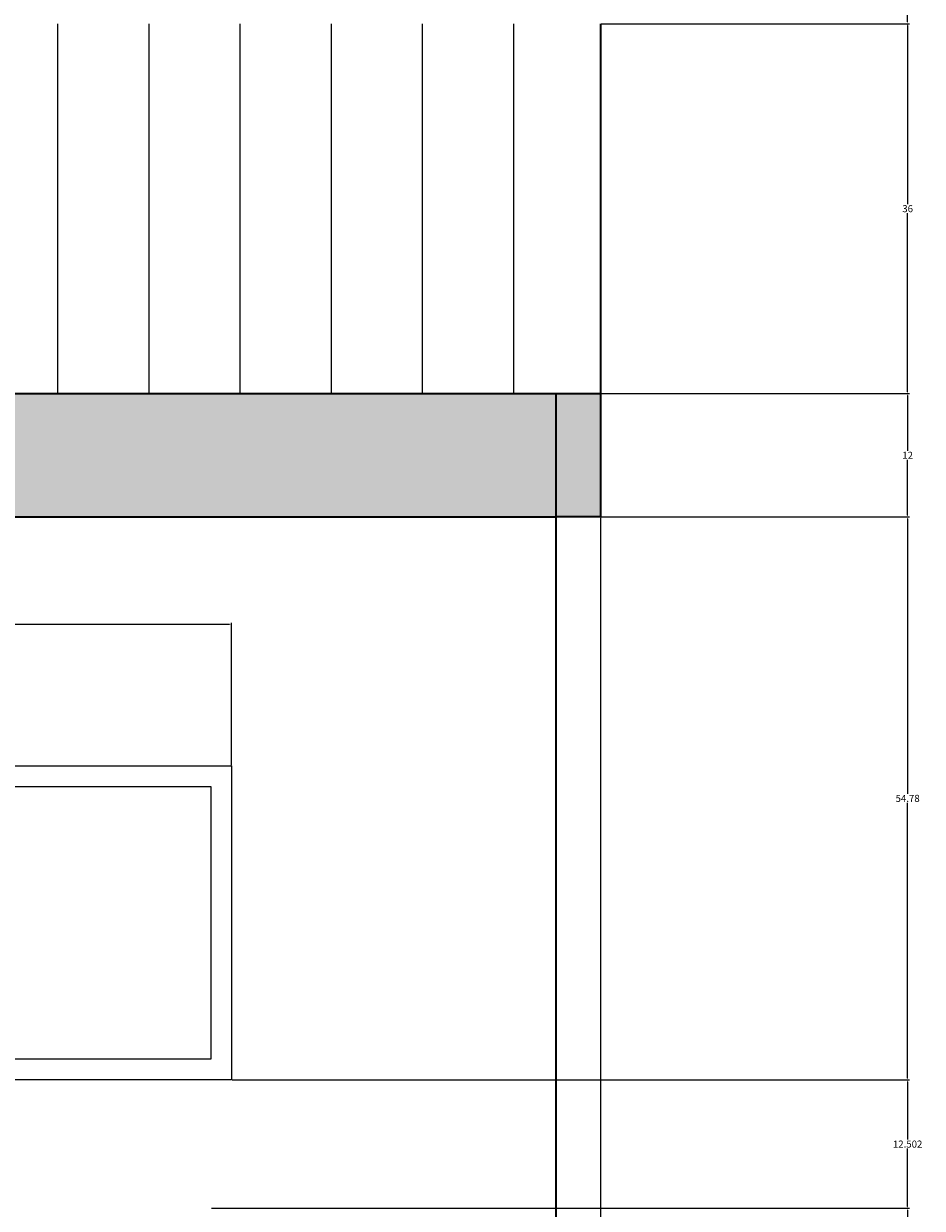
# Model space of a CAD drawing. Units: inches. Extents: x -145 to 510, y 5 to 386.
# Tile 24 of 25: x 423 to 510, y 157 to 272. Entities that reach past the tile are written whole.
import ezdxf

# ---------------------------------------------------------------- set-up
doc = ezdxf.new("R2010")
doc.units = ezdxf.units.IN
doc.header["$MEASUREMENT"] = 0
for name, color, linetype, lineweight in [('A-ANNO-DIMS', 2, 'Continuous', 18), ('A-ELEV', 7, 'Continuous', 35), ('A-ELEV-PATT', 8, 'Continuous', 13), ('A-GLAZ', 4, 'Continuous', 25)]:
    doc.layers.add(name, color=color, linetype=linetype, lineweight=lineweight)
doc.styles.get("Standard").update_dxf_attribs({"font": 'arial.ttf'})
doc.dimstyles.get("Standard").update_dxf_attribs({"dimtxt": 0.6875, "dimasz": 0.18, "dimexe": 0.18, "dimexo": 0.0625, "dimgap": 0.09, "dimtad": 0, "dimtih": 1, "dimtoh": 1, "dimdec": 4, "dimzin": 0, "dimdsep": 46, "dimlunit": 4, "dimtxsty": 'Standard', "dimcen": 0.09, "dimadec": 0, "dimazin": 0, "dimtfac": 1, "dimtdec": 4, "dimtofl": 0, "dimtmove": 0, "dimatfit": 3, "dimfxl": 1, "dimtolj": 1, "dimtzin": 0, "dimarcsym": 0})

# ---------------------------------------------------------------- blocks, each defined once
blk = doc.blocks.new('WIN-2200')
for points in [[(0, 30.55), (91.67, 30.55), (91.67, 0), (0, 0)], [(2, 28.55), (89.67, 28.55), (89.67, 2), (2, 2)]]:
    blk.add_lwpolyline(points, close=True)
blk = doc.blocks.new('*D5')
at = {"layer": 'A-ANNO-DIMS', "color": 0, "lineweight": -2, "transparency": 16777216}
for p, q in [((351.23, 199.73), (351.23, 213.6)), ((351.41, 213.42), (392.2, 213.42)), ((442.72, 213.42), (401.94, 213.42)), ((442.9, 199.73), (442.9, 213.6))]:
    blk.add_line(p, q, dxfattribs=at)
at = {"layer": 'A-ANNO-DIMS', "color": 0, "transparency": 16777216}
for points in [[(351.41, 213.45), (351.41, 213.39), (351.23, 213.42)], [(442.72, 213.45), (442.72, 213.39), (442.9, 213.42)]]:
    blk.add_solid(points, dxfattribs=at)
at = {"layer": 'Defpoints', "color": 0, "transparency": 16777216}
for p in [(442.9, 213.42), (351.23, 199.67), (442.9, 199.67)]:
    blk.add_point(p, dxfattribs=at)
at = {"layer": 'A-ANNO-DIMS', "color": 0, "transparency": 16777216, "insert": (397.07, 213.42), "char_height": 0.6875, "attachment_point": 5}
blk.add_mtext('\\A1;WINDOW W1 92 TYP.', dxfattribs=at)
blk = doc.blocks.new('*D19')
at = {"layer": 'A-ANNO-DIMS', "color": 0, "lineweight": -2, "transparency": 16777216}
for p, q in [((478.76, 355.89), (-144.05, 355.89)), ((-143.87, 355.71), (-143.87, 218.33)), ((-143.87, 80.07), (-143.87, 217.45)), ((-114.04, 79.89), (-144.05, 79.89))]:
    blk.add_line(p, q, dxfattribs=at)
at = {"layer": 'A-ANNO-DIMS', "color": 0, "transparency": 16777216}
for points in [[(-143.9, 355.71), (-143.84, 355.71), (-143.87, 355.89)], [(-143.9, 80.07), (-143.84, 80.07), (-143.87, 79.89)]]:
    blk.add_solid(points, dxfattribs=at)
at = {"layer": 'Defpoints', "color": 0, "transparency": 16777216}
for p in [(-143.87, 355.89), (478.83, 355.89), (-113.97, 79.89)]:
    blk.add_point(p, dxfattribs=at)
at = {"layer": 'A-ANNO-DIMS', "color": 0, "transparency": 16777216, "insert": (-143.87, 217.89), "char_height": 0.688, "attachment_point": 5}
blk.add_mtext('\\A1;276', dxfattribs=at)
blk = doc.blocks.new('*D32')
at = {"layer": 'A-ANNO-DIMS', "color": 0, "lineweight": -2, "transparency": 16777216}
for p, q in [((440.96, 156.61), (508.91, 156.61)), ((508.73, 156.43), (508.73, 136.37)), ((508.73, 115.44), (508.73, 135.49)), ((440.96, 115.26), (508.91, 115.26))]:
    blk.add_line(p, q, dxfattribs=at)
at = {"layer": 'A-ANNO-DIMS', "color": 0, "transparency": 16777216}
for points in [[(508.7, 156.43), (508.76, 156.43), (508.73, 156.61)], [(508.7, 115.44), (508.76, 115.44), (508.73, 115.26)]]:
    blk.add_solid(points, dxfattribs=at)
at = {"layer": 'Defpoints', "color": 0, "transparency": 16777216}
for p in [(440.9, 156.61), (508.73, 156.61), (440.9, 115.26)]:
    blk.add_point(p, dxfattribs=at)
at = {"layer": 'A-ANNO-DIMS', "color": 0, "transparency": 16777216, "insert": (508.73, 135.93), "char_height": 0.688, "attachment_point": 5}
blk.add_mtext('\\A1;41.35', dxfattribs=at)
blk = doc.blocks.new('*D33')
at = {"layer": 'A-ANNO-DIMS', "color": 0, "lineweight": -2, "transparency": 16777216}
for p, q in [((442.96, 169.11), (508.91, 169.11)), ((508.73, 168.93), (508.73, 163.3)), ((508.73, 156.79), (508.73, 162.42)), ((440.96, 156.61), (508.91, 156.61))]:
    blk.add_line(p, q, dxfattribs=at)
at = {"layer": 'A-ANNO-DIMS', "color": 0, "transparency": 16777216}
for points in [[(508.7, 168.93), (508.76, 168.93), (508.73, 169.11)], [(508.7, 156.79), (508.76, 156.79), (508.73, 156.61)]]:
    blk.add_solid(points, dxfattribs=at)
at = {"layer": 'Defpoints', "color": 0, "transparency": 16777216}
for p in [(442.9, 169.11), (508.73, 169.11), (440.9, 156.61)]:
    blk.add_point(p, dxfattribs=at)
at = {"layer": 'A-ANNO-DIMS', "color": 0, "transparency": 16777216, "insert": (508.73, 162.86), "char_height": 0.688, "attachment_point": 5}
blk.add_mtext('\\A1;12.502', dxfattribs=at)
blk = doc.blocks.new('*D34')
at = {"layer": 'A-ANNO-DIMS', "color": 0, "lineweight": -2, "transparency": 16777216}
for p, q in [((478.89, 223.89), (508.91, 223.89)), ((508.73, 223.71), (508.73, 196.94)), ((508.73, 169.29), (508.73, 196.06)), ((442.96, 169.11), (508.91, 169.11))]:
    blk.add_line(p, q, dxfattribs=at)
at = {"layer": 'A-ANNO-DIMS', "color": 0, "transparency": 16777216}
for points in [[(508.7, 223.71), (508.76, 223.71), (508.73, 223.89)], [(508.7, 169.29), (508.76, 169.29), (508.73, 169.11)]]:
    blk.add_solid(points, dxfattribs=at)
at = {"layer": 'Defpoints', "color": 0, "transparency": 16777216}
for p in [(478.83, 223.89), (508.73, 223.89), (442.9, 169.11)]:
    blk.add_point(p, dxfattribs=at)
at = {"layer": 'A-ANNO-DIMS', "color": 0, "transparency": 16777216, "insert": (508.73, 196.5), "char_height": 0.688, "attachment_point": 5}
blk.add_mtext('\\A1;54.78', dxfattribs=at)
blk = doc.blocks.new('*D35')
at = {"layer": 'A-ANNO-DIMS', "color": 0, "lineweight": -2, "transparency": 16777216}
for p, q in [((478.89, 235.89), (508.91, 235.89)), ((508.73, 235.71), (508.73, 230.33)), ((508.73, 224.07), (508.73, 229.46)), ((478.89, 223.89), (508.91, 223.89))]:
    blk.add_line(p, q, dxfattribs=at)
at = {"layer": 'A-ANNO-DIMS', "color": 0, "transparency": 16777216}
for points in [[(508.7, 235.71), (508.76, 235.71), (508.73, 235.89)], [(508.7, 224.07), (508.76, 224.07), (508.73, 223.89)]]:
    blk.add_solid(points, dxfattribs=at)
at = {"layer": 'Defpoints', "color": 0, "transparency": 16777216}
for p in [(478.83, 235.89), (508.73, 235.89), (478.83, 223.89)]:
    blk.add_point(p, dxfattribs=at)
at = {"layer": 'A-ANNO-DIMS', "color": 0, "transparency": 16777216, "insert": (508.73, 229.89), "char_height": 0.688, "attachment_point": 5}
blk.add_mtext('\\A1;12', dxfattribs=at)
blk = doc.blocks.new('*D36')
at = {"layer": 'A-ANNO-DIMS', "color": 0, "lineweight": -2, "transparency": 16777216}
for p, q in [((478.89, 271.89), (508.91, 271.89)), ((508.73, 271.71), (508.73, 254.33)), ((508.73, 236.07), (508.73, 253.45)), ((478.89, 235.89), (508.91, 235.89))]:
    blk.add_line(p, q, dxfattribs=at)
at = {"layer": 'A-ANNO-DIMS', "color": 0, "transparency": 16777216}
for points in [[(508.7, 271.71), (508.76, 271.71), (508.73, 271.89)], [(508.7, 236.07), (508.76, 236.07), (508.73, 235.89)]]:
    blk.add_solid(points, dxfattribs=at)
at = {"layer": 'Defpoints', "color": 0, "transparency": 16777216}
for p in [(478.83, 271.89), (508.73, 271.89), (478.83, 235.89)]:
    blk.add_point(p, dxfattribs=at)
at = {"layer": 'A-ANNO-DIMS', "color": 0, "transparency": 16777216, "insert": (508.73, 253.89), "char_height": 0.688, "attachment_point": 5}
blk.add_mtext('\\A1;36', dxfattribs=at)
blk = doc.blocks.new('*D37')
at = {"layer": 'A-ANNO-DIMS', "color": 0, "lineweight": -2, "transparency": 16777216}
for p, q in [((442.96, 301.88), (508.91, 301.88)), ((508.73, 301.7), (508.73, 287.33)), ((508.73, 272.07), (508.73, 286.45)), ((478.89, 271.89), (508.91, 271.89))]:
    blk.add_line(p, q, dxfattribs=at)
at = {"layer": 'A-ANNO-DIMS', "color": 0, "transparency": 16777216}
for points in [[(508.7, 301.7), (508.76, 301.7), (508.73, 301.88)], [(508.7, 272.07), (508.76, 272.07), (508.73, 271.89)]]:
    blk.add_solid(points, dxfattribs=at)
at = {"layer": 'Defpoints', "color": 0, "transparency": 16777216}
for p in [(442.9, 301.88), (508.73, 301.88), (478.83, 271.89)]:
    blk.add_point(p, dxfattribs=at)
at = {"layer": 'A-ANNO-DIMS', "color": 0, "transparency": 16777216, "insert": (508.73, 286.89), "char_height": 0.688, "attachment_point": 5}
blk.add_mtext('\\A1;29.99', dxfattribs=at)
blk = doc.blocks.new('*D49')
at = {"layer": 'A-ANNO-DIMS', "color": 0, "lineweight": -2, "transparency": 16777216}
for p, q in [((474.49, 223.83), (474.49, 5.19)), ((478.83, 223.83), (478.83, 5.19)), ((474.67, 5.37), (475.39, 5.37)), ((478.65, 5.37), (477.92, 5.37))]:
    blk.add_line(p, q, dxfattribs=at)
at = {"layer": 'A-ANNO-DIMS', "color": 0, "transparency": 16777216}
for points in [[(474.67, 5.4), (474.67, 5.34), (474.49, 5.37)], [(478.65, 5.4), (478.65, 5.34), (478.83, 5.37)]]:
    blk.add_solid(points, dxfattribs=at)
at = {"layer": 'Defpoints', "color": 0, "transparency": 16777216}
for p in [(474.49, 223.89), (478.83, 223.89), (478.83, 5.37)]:
    blk.add_point(p, dxfattribs=at)
at = {"layer": 'A-ANNO-DIMS', "color": 0, "transparency": 16777216, "insert": (476.66, 5.37), "char_height": 0.688, "attachment_point": 5}
blk.add_mtext('\\A1;4.337', dxfattribs=at)

msp = doc.modelspace()

# ---------------------------------------------------------------- hatches: boundary and pattern name
at = {"layer": 'A-ELEV-PATT'}
h = msp.add_hatch(color=256, dxfattribs=at)
h.dxf.hatch_style = 1
h.paths.add_polyline_path([(334.4402, 341.168), (69.7763, 341.168), (69.7763, 327.6093), (334.4402, 327.6093)])
h.paths.add_polyline_path([(69.7763, 341.168), (34.2706, 341.168), (34.2706, 327.6093), (69.7763, 327.6093)])
h.paths.add_polyline_path([(317.2273, 188.3087), (210.7973, 188.3087), (210.7973, 178.0195), (317.2273, 178.0195)])
h.paths.add_polyline_path([(474.4893, 235.8905), (317.2273, 235.8905), (317.2273, 223.8905), (474.4893, 223.8905)])
h.paths.add_polyline_path([(317.2273, 235.8905), (309.4739, 235.8905), (309.4739, 223.8905), (317.2273, 223.8905)])
h.paths.add_polyline_path([(478.8263, 235.8905), (474.4893, 235.8905), (474.4893, 223.8905), (478.8263, 223.8905)])
h = msp.add_hatch(dxfattribs=at)
h.set_pattern_fill('ANSI31', color=256, scale=71, angle=45)
h.paths.add_polyline_path([(478.8263, 271.8905), (309.4739, 271.8905), (309.4739, 259.8905), (309.4739, 235.8905), (317.2273, 235.8905), (474.4893, 235.8905), (478.8263, 235.8905)])

# ---------------------------------------------------------------- linework, layer by layer
at = {"layer": 'A-ELEV'}
for p, q in [((478.8263, 271.8905), (478.8263, 235.8905)), ((317.2273, 235.8905), (474.4893, 235.8905)), ((474.4893, 235.8905), (474.4893, 223.8905)), ((474.4893, 235.8905), (478.8263, 235.8905)), ((478.8263, 235.8905), (478.8263, 223.8905)), ((317.2273, 223.8905), (474.4893, 223.8905)), ((474.4893, 223.8905), (474.4893, 79.8905)), ((478.8263, 223.8905), (474.4893, 223.8905))]:
    msp.add_line(p, q, dxfattribs=at)

# ---------------------------------------------------------------- block references
at = {"layer": 'A-GLAZ'}
msp.add_blockref('WIN-2200', (351.234, 169.112), dxfattribs=at)

# ---------------------------------------------------------------- dimensions: what is measured, and where the dimension line sits
at = {"layer": 'A-ANNO-DIMS'}
for base, p1, p2, override, picture, middle in [((-143.8737, 355.8905), (-113.9737, 79.8905), (478.8263, 355.8905), {"dimdec": 0, "dimlfac": 1, "dimrnd": 0, "dimzin": 0, "dimdsep": 46, "dimlunit": 2}, '*D19', (-143.8737, 217.8905)), ((508.7263, 301.8821), (478.8263, 271.8905), (442.9009, 301.8821), {"dimdec": 2, "dimlfac": 1, "dimrnd": 0, "dimzin": 0, "dimdsep": 46, "dimlunit": 2}, '*D37', (508.7263, 286.8863)), ((508.7263, 271.8905), (478.8263, 235.8905), (478.8263, 271.8905), {"dimdec": 0, "dimlfac": 1, "dimrnd": 0, "dimzin": 0, "dimdsep": 46, "dimlunit": 2}, '*D36', (508.7263, 253.8905)), ((508.7263, 235.8905), (478.8263, 223.8905), (478.8263, 235.8905), {"dimdec": 0, "dimlfac": 1, "dimrnd": 0, "dimzin": 0, "dimdsep": 46, "dimlunit": 2}, '*D35', (508.7263, 229.8905)), ((508.7263, 223.8905), (442.9009, 169.1117), (478.8263, 223.8905), {"dimdec": 2, "dimlfac": 1, "dimrnd": 0, "dimzin": 0, "dimdsep": 46, "dimlunit": 2}, '*D34', (508.7263, 196.5011)), ((508.7263, 169.1117), (440.9009, 156.6093), (442.9009, 169.1117), {"dimdec": 3, "dimlfac": 1, "dimrnd": 0, "dimzin": 0, "dimdsep": 46, "dimlunit": 2}, '*D33', (508.7263, 162.8605)), ((508.7263, 156.6093), (440.9009, 115.2574), (440.9009, 156.6093), {"dimdec": 2, "dimlfac": 1, "dimrnd": 0, "dimzin": 0, "dimdsep": 46, "dimlunit": 2}, '*D32', (508.7263, 135.9333))]:
    dim = msp.add_linear_dim(base=base, p1=p1, p2=p2, angle=90, dimstyle='Standard', override=override, dxfattribs=at)
    dim.commit()
    dim.dimension.update_dxf_attribs({"geometry": picture, "text_midpoint": middle})
dim = msp.add_linear_dim(base=(478.8263, 5.3738), p1=(474.4893, 223.8905), p2=(478.8263, 223.8905), dimstyle='Standard', override={"dimdec": 3, "dimlfac": 1, "dimrnd": 0, "dimzin": 0, "dimdsep": 46, "dimlunit": 2}, dxfattribs=at)
dim.commit()
dim.dimension.update_dxf_attribs({"geometry": '*D49', "text_midpoint": (476.6578, 5.3738)})
dim = msp.add_linear_dim(base=(442.9009, 213.4154), p1=(351.234, 199.6654), p2=(442.9009, 199.6654), text='WINDOW W1 <> TYP.', dimstyle='Standard', override={"dimdec": 0, "dimlfac": 1, "dimrnd": 0, "dimzin": 0, "dimdsep": 46, "dimlunit": 2}, dxfattribs=at)
dim.commit()
dim.dimension.update_dxf_attribs({"geometry": '*D5', "text_midpoint": (397.0675, 213.4154)})

doc.saveas('drawing.dxf')
